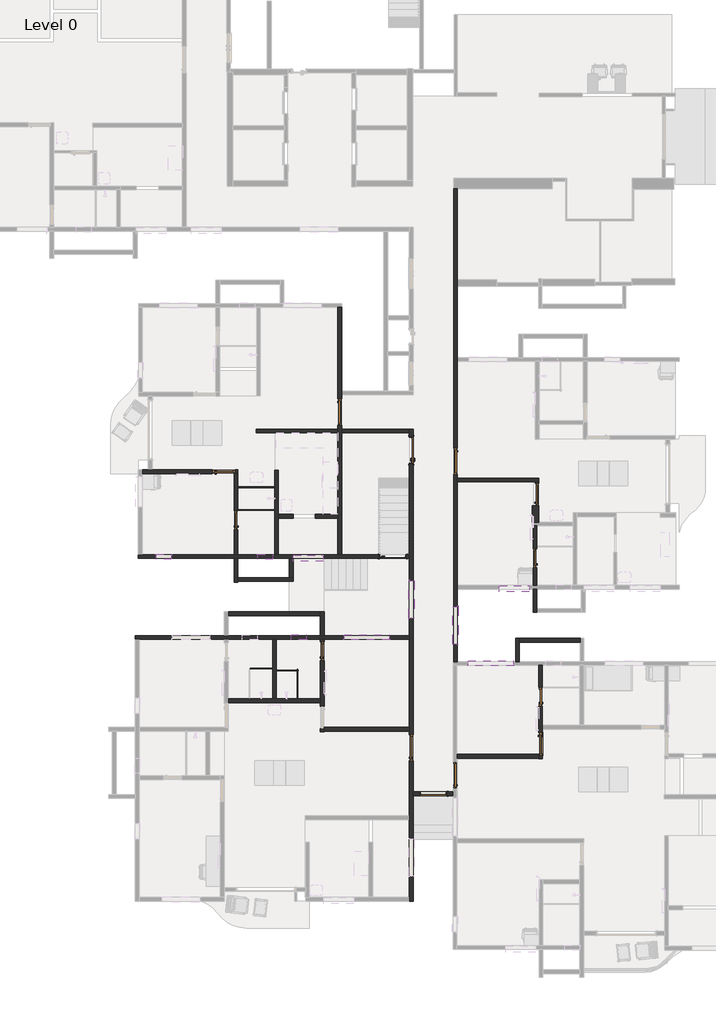
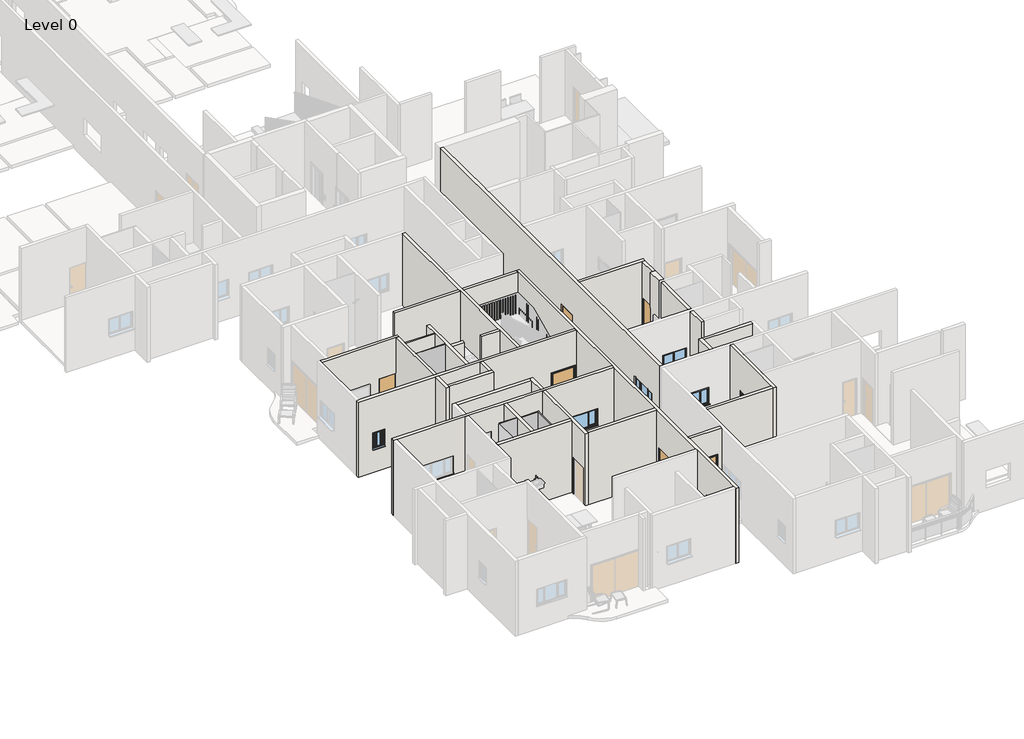
# One storey, part 2 of 14: 28 walls, 14 doors, 9 windows, 4 plates.
# Revit data of these elements (continued)
# Type "Windows_Tpl_Variable_Casement : 2'" (continued)
#   Wrap Layers (Ext) from Ext = 102.5 mm
#   Window Board Projection = 25 mm
#   Window Board Extension = 25 mm
#   Visual Light Transmittance = 0.9
#   Solar Heat Gain Coefficient = 0.78
#   Rough Width = 609.6 mm
#   Rough Height = 910 mm
#   Height = 910 mm
#   Width = 609.6 mm
#   Heat Transfer Coefficient (U) = 3.6886 W/(m²·K)
#   Glazing Thickness = 24 mm
#   FrameOffset - External = 50 mm
#   Frame Depth = 65 mm
#   Default Head Height = 2110 mm
#   Cill Depth = 87.5 mm
#   Cavity Closer Width = 50 mm
#   Cavity Closer Offset from Ext = 102.5 mm
#   Cavity Closer Depth = 85 mm
#   Casement Width = 450 mm
#   Vis - Cavity Closers = yes
#   Define Thermal Properties by = 1
#   Material Trim = Window Frame
#   Material Glass = Glass
#   Material Frame = Window Frame
#   Wall Closure = (empty or 0)
# Type "Windows_Tpl_Variable_Casement : 5'"
#   Type Mark = "83"
#   Operation = "TriplePanelVertical"
#   Construction Type Id = "GSP4R"
#   Manufacturer = "Revit"
#   Keynote = "L10"
#   Analytic Construction = "1/8 in Pilkington single glazing"
#   Wrap Layers (Int) from Ext = 177.5 mm
#   Wrap Layers (Ext) from Ext = 102.5 mm
#   Window Board Projection = 25 mm
#   Window Board Extension = 25 mm
#   Visual Light Transmittance = 0.9
#   Solar Heat Gain Coefficient = 0.78
#   Rough Width = 1524 mm
#   Rough Height = 910 mm
#   Height = 910 mm
#   Width = 1524 mm
#   Heat Transfer Coefficient (U) = 3.6886 W/(m²·K)
#   Glazing Thickness = 24 mm
#   FrameOffset - External = 50 mm
#   Frame Depth = 65 mm
#   Default Head Height = 2110 mm
#   Cill Depth = 87.5 mm
#   Cavity Closer Width = 50 mm
#   Cavity Closer Offset from Ext = 102.5 mm
#   Cavity Closer Depth = 85 mm
#   Casement Width = 450 mm
#   Vis - Cavity Closers = yes
#   Define Thermal Properties by = 1
#   Material Trim = Window Frame
#   Material Glass = Glass
#   Material Frame = Window Frame
#   Wall Closure = (empty or 0)
# Type "Windows_Tpl_Variable_Casement : 6'"
#   Type Mark = "84"
#   Operation = "TriplePanelVertical"
#   Construction Type Id = "GSP4R"
#   Manufacturer = "Revit"
#   Keynote = "L10"
#   Analytic Construction = "1/8 in Pilkington single glazing"
#   Wrap Layers (Int) from Ext = 177.5 mm
#   Wrap Layers (Ext) from Ext = 102.5 mm
#   Window Board Projection = 25 mm
#   Window Board Extension = 25 mm
#   Visual Light Transmittance = 0.9
#   Solar Heat Gain Coefficient = 0.78
#   Rough Width = 1828.8 mm
#   Rough Height = 910 mm
#   Height = 910 mm
#   Width = 1828.8 mm
#   Heat Transfer Coefficient (U) = 3.6886 W/(m²·K)
#   Glazing Thickness = 24 mm
#   FrameOffset - External = 50 mm
#   Frame Depth = 65 mm
#   Default Head Height = 2110 mm
#   Cill Depth = 87.5 mm
#   Cavity Closer Width = 50 mm
#   Cavity Closer Offset from Ext = 102.5 mm
#   Cavity Closer Depth = 85 mm
#   Casement Width = 450 mm
#   Vis - Cavity Closers = yes
#   Define Thermal Properties by = 1
#   Material Trim = Window Frame
#   Material Glass = Glass
#   Material Frame = Window Frame
#   Wall Closure = (empty or 0)
# Elements 1, 2, 3, 4 (IfcDoor, "Doors_ExtSgl_Flush : D1")
#   Phase Created = New Construction
#   Materials on its faces: "Door - Handle", "Door - Frame/Mullion", "Door - Panel"
# Elements 5, 6, 7 (IfcDoor, "Doors_ExtSgl_Flush : D2")
#   Phase Created = New Construction
#   Materials on its faces: "Door - Handle", "Door - Frame/Mullion", "Door - Panel"
# Elements 8, 9, 10, 11 (IfcDoor, "Doors_ExtSgl_Flush : D3")
#   Phase Created = New Construction
#   Materials on its faces: "Door - Handle", "Door - Frame/Mullion", "Door - Panel"
# Elements 12, 13, 14 (IfcDoor, "Doors_IntSgl : 3.75'")
#   Phase Created = New Construction
#   Materials on its faces: "Door - Architrave", "Door - Handle", "Door - Frame/Mullion (1)", "Door - Panel"
# Elements 15, 16, 17, 18 (IfcPlate, "System Panel : Glazed")
#   Phase Created = New Construction
#   Materials on its faces: "Glass"
# Elements 19, 20, 21, 22, 23, 24, 25, 26, 27, 28, 29, 30, 31, 32, 33, 34, 35, 36, 37, 38, 39, 40, 41, 42, 43, 44 (IfcWall, "W1")
#   Top Offset = 0 mm
#   Base Offset = 0 mm
#   wall height = 4000 mm
#   Phase Created = New Construction
#   Base Constraint = Level 0
#   Top Constraint = Level 1
#   Materials on its faces: "Brick, Common"
# Element 45 (IfcWall, "W2")
#   Top Offset = 0 mm
#   Base Offset = 0 mm
#   wall height = 4000 mm
#   Phase Created = New Construction
#   Base Constraint = Level 0
#   Top Constraint = Level 1
#   Materials on its faces: "Brick, Common"
# Element 46 (IfcWall, "W3")
#   Top Offset = 0 mm
#   Base Offset = 0 mm
#   wall height = 4000 mm
#   Phase Created = New Construction
#   Base Constraint = Level 0
#   Top Constraint = Level 1
#   Materials on its faces: "Brick, Common"
# Element 47 (IfcWindow, "Windows_Concept_Plain_Dbl : 4'")
#   Mark = "24"
#   Phase Created = New Construction
#   Materials on its faces: "Window Frame", "Glass"
# Element 48 (IfcWindow, "Windows_Concept_Plain_Dbl : 4'")
#   Mark = "66"
#   Phase Created = New Construction
#   Materials on its faces: "Window Frame", "Glass"
# Element 49 (IfcWindow, "Windows_Sgl_Plain : 2'")
#   Mark = "6"
#   Phase Created = New Construction
#   Materials on its faces: "Window Frame", "Glass"
# Element 50 (IfcWindow, "Windows_Sgl_Plain : 2'")
#   Mark = "67"
#   Phase Created = New Construction
#   Materials on its faces: "Window Frame", "Glass"
# Element 51 (IfcWindow, "Windows_Tpl_Variable_Casement : 2'")
#   Mark = "64"
#   Phase Created = New Construction
#   Materials on its faces: "Window Frame", "Glass"
# Element 52 (IfcWindow, "Windows_Tpl_Variable_Casement : 5'")
#   Mark = "69"
#   Phase Created = New Construction
#   Materials on its faces: "Window Frame", "Glass"
# Element 53 (IfcWindow, "Windows_Tpl_Variable_Casement : 5'")
#   Mark = "70"
#   Phase Created = New Construction
#   Materials on its faces: "Window Frame", "Glass"
# Element 54 (IfcWindow, "Windows_Tpl_Variable_Casement : 6'")
#   Mark = "9"
#   Phase Created = New Construction
#   Materials on its faces: "Window Frame", "Glass"
# Element 55 (IfcWindow, "Windows_Tpl_Variable_Casement : 6'")
#   Mark = "15"
#   Phase Created = New Construction
#   Materials on its faces: "Window Frame", "Glass"
# Materials
#   "Door - Panel": class "Wood", colour RGB 210 159 95, transparency 0, Keynote = "L20", Cost = 0
#   "Door - Frame/Mullion": class "Wood", colour RGB 212 179 113, transparency 0, Keynote = "L20", Cost = 0
#   "Door - Handle": colour RGB 0 0 0, transparency 0, Keynote = "P21", Cost = 0
#   "Door - Frame/Mullion (1)": class "Wood", colour RGB 212 179 113, transparency 0, Keynote = "L20", Cost = 0
#   "Door - Architrave": class "Wood", colour RGB 154 90 5, transparency 0, Keynote = "P20", Cost = 0
#   "Brick, Common": class "Masonry", colour RGB 170 100 105, transparency 0, Description = "Common brick", Cost = 0
#   "Window Frame": colour RGB 249 249 249, transparency 0, Keynote = "L10", Cost = 0
#   "Glass": class "Glass", colour RGB 0 128 192, transparency 0.9, Description = "Soda Lime Glass", Cost = 0
